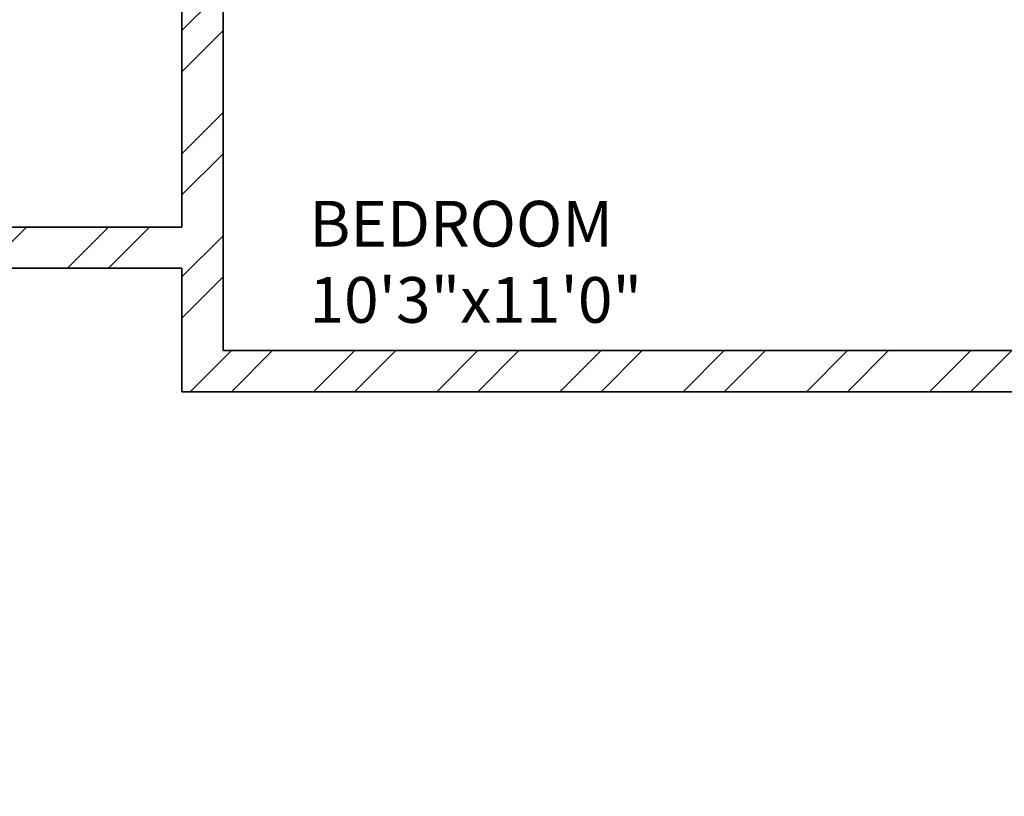
# Model space of a CAD drawing. Units: inches. Extents: x 1885 to 2748, y 783 to 2421.
# Tile 90 of 117: x 2341 to 2449, y 2167 to 2252. Entities that reach past the tile are written whole.
import ezdxf

# ---------------------------------------------------------------- set-up
doc = ezdxf.new("R2010")
doc.units = ezdxf.units.IN
doc.layers.add('A-AREA-IDEN', color=7, linetype='Continuous', lineweight=18)
doc.layers.add('A-WALL', color=7, linetype='Continuous', lineweight=35)
doc.layers.add('A-WALL-PATT', color=85, linetype='Continuous', lineweight=13, true_color=0x58ba48)
doc.styles.get("Standard").update_dxf_attribs({"font": 'arial.ttf'})

msp = doc.modelspace()

# ---------------------------------------------------------------- hatches: boundary and pattern name
at = {"layer": 'A-WALL-PATT'}
h = msp.add_hatch(dxfattribs=at)
h.set_pattern_fill('ANSI32', color=256)
h.paths.add_polyline_path([(2007.77, 2318.01), (1980.77, 2318.01), (1980.77, 2281.22), (1985.27, 2281.22), (1985.27, 2313.51), (2007.77, 2313.51), (2007.77, 2315.76)])
h.paths.add_polyline_path([(2094.32, 2318.01), (2067.77, 2318.01), (2067.77, 2313.51), (2094.32, 2313.51), (2094.32, 2315.76)])
h.paths.add_polyline_path([(2131.37, 2315.76), (2131.37, 2318.01), (2131.19, 2318.01), (2112.61, 2318.01), (2112.61, 2313.51), (2117.27, 2313.51), (2117.27, 2255.2), (2121.77, 2255.2), (2121.77, 2313.51), (2131.37, 2313.51)])
h.paths.add_polyline_path([(2190.51, 2318.01), (2155.37, 2318.01), (2155.37, 2313.51), (2169.77, 2313.51), (2169.77, 2229.51), (2121.77, 2229.51), (2121.77, 2233.45), (2119.52, 2233.45), (2117.27, 2233.45), (2117.27, 2201.1), (2121.77, 2201.1), (2121.77, 2225.01), (2169.77, 2225.01), (2169.77, 2165.01), (2306.27, 2165.01), (2306.27, 2066.01), (2310.77, 2066.01), (2344.27, 2066.01), (2486.27, 2066.01), (2486.27, 1886.01), (2483.02, 1886.01), (2483.02, 1881.51), (2486.27, 1881.51), (2486.27, 1880.68), (2490.77, 1880.68), (2490.77, 2070.51), (2344.27, 2070.51), (2310.77, 2070.51), (2310.77, 2165.01), (2310.77, 2173.64), (2308.52, 2173.64), (2306.27, 2173.64), (2306.27, 2169.51), (2174.27, 2169.51), (2174.27, 2313.51), (2190.51, 2313.51), (2190.51, 2315.76)])
h.paths.add_polyline_path([(1985.27, 2221.22), (1980.77, 2221.22), (1980.77, 2165.01), (1992.77, 2165.01), (1992.77, 2141.93), (1997.27, 2141.93), (1997.27, 2165.01), (2117.27, 2165.01), (2117.27, 2163.13), (2121.77, 2163.13), (2121.77, 2172.73), (2119.52, 2172.73), (2117.27, 2172.73), (2117.27, 2169.51), (1985.27, 2169.51)])
h.paths.add_polyline_path([(1997.27, 2105.93), (1992.77, 2105.93), (1992.77, 2070.51), (2016.77, 2070.51), (2016.77, 2059.12), (2019.02, 2059.12), (2021.27, 2059.12), (2021.27, 2070.51), (2117.27, 2070.51), (2117.27, 2022.51), (2114.42, 2022.51), (2114.42, 2018.01), (2123.63, 2018.01), (2123.63, 2020.26), (2123.63, 2022.51), (2121.77, 2022.51), (2121.77, 2142.59), (2119.52, 2142.59), (2117.27, 2142.59), (2117.27, 2075.01), (1997.27, 2075.01)])
h.paths.add_polyline_path([(2092.03, 2020.26), (2092.03, 2022.51), (2021.27, 2022.51), (2021.27, 2035.12), (2016.77, 2035.12), (2016.77, 2018.01), (2016.77, 1978.78), (2021.27, 1978.78), (2021.27, 2018.01), (2092.03, 2018.01)])
h.paths.add_polyline_path([(2260.94, 2022.51), (2153.1, 2022.51), (2153.1, 2020.26), (2153.1, 2018.01), (2155.27, 2018.01), (2155.27, 1886.01), (2107.63, 1886.01), (2107.63, 1881.51), (2182.91, 1881.51), (2182.91, 1883.76), (2182.91, 1886.01), (2159.77, 1886.01), (2159.77, 2018.01), (2260.94, 2018.01), (2260.94, 2020.26)])
h.paths.add_polyline_path([(2047.63, 1883.76), (2047.63, 1886.01), (2021.27, 1886.01), (2021.27, 1918.78), (2019.02, 1918.78), (2016.77, 1918.78), (2016.77, 1881.51), (2047.63, 1881.51)])
h.paths.add_polyline_path([(2306.36, 1883.76), (2306.36, 1886.01), (2296.27, 1886.01), (2296.27, 1982.01), (2316.54, 1982.01), (2316.54, 1984.26), (2316.54, 1986.51), (2296.27, 1986.51), (2296.27, 2022.51), (2289.28, 2022.51), (2289.28, 2018.01), (2291.77, 2018.01), (2291.77, 1886.01), (2242.91, 1886.01), (2242.91, 1881.51), (2306.36, 1881.51)], flags=17)
h.paths.add_polyline_path([(1985.27, 1843.01), (2021.6, 1843.01), (2021.53, 1845.44), (2021.48, 1847.51), (1980.77, 1847.51), (1980.77, 1809.45), (1985.27, 1809.45)])
h.paths.add_polyline_path([(2131.48, 1845.26), (2131.48, 1847.51), (2081.53, 1847.51), (2081.53, 1843.01), (2117.27, 1843.01), (2117.27, 1784.15), (2119.52, 1784.15), (2121.77, 1784.15), (2121.77, 1843.01), (2131.48, 1843.01)])
h.paths.add_polyline_path([(2203.89, 1847.51), (2155.48, 1847.51), (2155.48, 1843.01), (2169.77, 1843.01), (2169.77, 1759.01), (2121.77, 1759.01), (2121.77, 1761.46), (2117.27, 1761.46), (2117.27, 1730.43), (2121.77, 1730.43), (2121.77, 1754.51), (2177.42, 1754.51), (2177.42, 1756.76), (2177.42, 1759.01), (2174.27, 1759.01), (2174.27, 1843.01), (2203.89, 1843.01)])
h.paths.add_polyline_path([(2335.55, 1845.26), (2335.55, 1847.51), (2239.89, 1847.51), (2239.89, 1843.01), (2306.27, 1843.01), (2306.27, 1759.01), (2199.49, 1759.01), (2199.49, 1754.51), (2310.77, 1754.51), (2310.77, 1843.01), (2335.55, 1843.01)])
h.paths.add_polyline_path([(2348.77, 2022.51), (2344.27, 2022.51), (2344.27, 1986.51), (2341.68, 1986.51), (2341.68, 1982.01), (2344.27, 1982.01), (2344.27, 1886.01), (2330.36, 1886.01), (2330.36, 1881.51), (2361.63, 1881.51), (2361.63, 1883.76), (2361.63, 1886.01), (2348.77, 1886.01)], flags=17)
h.paths.add_polyline_path([(2283.25, 2315.76), (2283.25, 2318.01), (2238.51, 2318.01), (2238.51, 2313.51), (2283.25, 2313.51)], flags=17)
h.paths.add_polyline_path([(2363.27, 2348.01), (2388.68, 2348.01), (2388.68, 2350.26), (2388.68, 2352.51), (2358.77, 2352.51), (2358.77, 2348.01), (2358.77, 2318.01), (2344.48, 2318.01), (2344.48, 2313.51), (2358.77, 2313.51), (2358.77, 2229.51), (2310.77, 2229.51), (2310.77, 2231.95), (2306.27, 2231.95), (2306.27, 2205.61), (2310.77, 2205.61), (2310.77, 2225.01), (2358.77, 2225.01), (2358.77, 2211.51), (2452.33, 2211.51), (2452.33, 2213.76), (2452.33, 2216.01), (2363.27, 2216.01), (2363.27, 2318.01)])
h.paths.add_polyline_path([(2310.77, 2313.51), (2320.48, 2313.51), (2320.48, 2315.76), (2320.48, 2318.01), (2302.73, 2318.01), (2302.73, 2313.51), (2306.27, 2313.51), (2306.27, 2251.08), (2310.77, 2251.08)], flags=17)
h.paths.add_polyline_path([(2490.77, 2352.51), (2486.27, 2352.51), (2448.68, 2352.51), (2448.68, 2348.01), (2486.27, 2348.01), (2486.27, 2318.01), (2486.27, 2216.01), (2481.78, 2216.01), (2481.78, 2211.51), (2486.27, 2211.51), (2486.27, 2165.01), (2493.29, 2165.01), (2493.29, 2167.26), (2493.29, 2169.51), (2490.77, 2169.51), (2490.77, 2313.51), (2494.43, 2313.51), (2494.43, 2318.01), (2490.77, 2318.01)])
h.paths.add_polyline_path([(2534.65, 2318.01), (2515.69, 2318.01), (2515.69, 2313.51), (2534.65, 2313.51), (2534.65, 2315.76)])
h.paths.add_polyline_path([(2618.27, 2318.01), (2594.65, 2318.01), (2594.65, 2313.51), (2613.77, 2313.51), (2613.77, 2281.71), (2618.27, 2281.71)])
h.paths.add_polyline_path([(2618.27, 2221.71), (2613.77, 2221.71), (2613.77, 2169.51), (2554.02, 2169.51), (2554.02, 2165.01), (2613.77, 2165.01), (2613.77, 2152.88), (2618.27, 2152.88)])
h.paths.add_polyline_path([(2618.27, 2128.88), (2616.02, 2128.88), (2613.77, 2128.88), (2613.77, 2117.01), (2529.77, 2117.01), (2529.77, 2165.01), (2532.85, 2165.01), (2532.85, 2169.51), (2522.87, 2169.51), (2522.87, 2165.01), (2525.27, 2165.01), (2525.27, 2117.01), (2525.27, 2112.51), (2525.27, 2108.58), (2529.77, 2108.58), (2529.77, 2112.51), (2613.77, 2112.51), (2613.77, 2080.19), (2618.27, 2080.19)])
h.paths.add_polyline_path([(2618.27, 2044.19), (2616.02, 2044.19), (2613.77, 2044.19), (2613.77, 2015.51), (2529.77, 2015.51), (2529.77, 2088.58), (2527.52, 2088.58), (2525.27, 2088.58), (2525.27, 2011.01), (2613.77, 2011.01), (2613.77, 1956.75), (2618.27, 1956.75)])
h.paths.add_polyline_path([(2618.27, 1881.51), (2618.27, 1896.75), (2613.77, 1896.75), (2613.77, 1881.51), (2613.77, 1847.51), (2592.71, 1847.51), (2592.71, 1843.01), (2613.77, 1843.01), (2613.77, 1765.01), (2613.77, 1760.51), (2609.62, 1760.51), (2609.62, 1756.01), (2613.77, 1756.01), (2613.77, 1660.01), (2608.54, 1660.01), (2608.54, 1655.51), (2613.77, 1655.51), (2613.77, 1508.16), (2618.27, 1508.16)])
h.paths.add_polyline_path([(2565.77, 1843.01), (2569, 1843.01), (2569, 1847.51), (2490.77, 1847.51), (2490.77, 1849.7), (2488.52, 1849.7), (2486.27, 1849.7), (2486.27, 1847.51), (2477.27, 1847.51), (2477.27, 1838.51), (2477.27, 1821.49), (2486.27, 1821.49), (2486.27, 1838.51), (2561.27, 1838.51), (2561.27, 1765.01), (2486.27, 1765.01), (2486.27, 1786.16), (2477.27, 1786.16), (2477.27, 1765.01), (2477.27, 1756.01), (2486.27, 1756.01), (2565.77, 1756.01), (2585.62, 1756.01), (2585.62, 1758.26), (2585.62, 1760.51), (2565.77, 1760.51), (2565.77, 1765.01)])
h.paths.add_polyline_path([(2486.27, 1651.01), (2561.27, 1651.01), (2561.27, 1567.01), (2486.27, 1567.01), (2486.27, 1591.32), (2477.27, 1591.32), (2477.27, 1567.01), (2477.27, 1558.01), (2477.27, 1555.44), (2481.77, 1555.44), (2481.77, 1558.01), (2568.65, 1558.01), (2568.65, 1560.26), (2568.65, 1562.51), (2565.77, 1562.51), (2565.77, 1655.51), (2584.54, 1655.51), (2584.54, 1657.76), (2584.54, 1660.01), (2565.77, 1660.01), (2486.27, 1660.01), (2477.27, 1660.01), (2477.27, 1651.01), (2477.27, 1632.99), (2486.27, 1632.99)])
h.paths.add_polyline_path([(2449.97, 1883.76), (2449.97, 1886.01), (2421.63, 1886.01), (2421.63, 1881.51), (2449.97, 1881.51)], flags=17)
h.paths.add_polyline_path([(2447.27, 1847.51), (2395.55, 1847.51), (2395.55, 1843.01), (2442.77, 1843.01), (2442.77, 1809.27), (2447.27, 1809.27)])
h.paths.add_polyline_path([(1985.27, 1749.45), (1980.77, 1749.45), (1980.77, 1694.5), (1985.27, 1694.5), (1985.27, 1694.51), (1986.9, 1694.51), (1986.9, 1697.78), (1986.9, 1699.01), (1985.27, 1699.01)])
h.paths.add_polyline_path([(2152.77, 1699.01), (2121.77, 1699.01), (2121.77, 1703.67), (2119.52, 1703.67), (2117.27, 1703.67), (2117.27, 1699.01), (2009.22, 1699.01), (2009.22, 1694.51), (2148.27, 1694.51), (2148.27, 1692.63), (2152.77, 1692.63)])
h.paths.add_polyline_path([(2016.27, 1694.51), (2011.77, 1694.51), (2011.77, 1558.01), (2040.81, 1558.01), (2040.81, 1560.26), (2040.81, 1562.51), (2016.27, 1562.51)])
h.paths.add_polyline_path([(2152.77, 1663.02), (2150.52, 1663.02), (2148.27, 1663.02), (2148.27, 1562.51), (2100.81, 1562.51), (2100.81, 1558.01), (2165.12, 1558.01), (2165.12, 1560.26), (2165.12, 1562.51), (2152.77, 1562.51), (2152.77, 1610.51), (2224.77, 1610.51), (2224.77, 1607.99), (2229.27, 1607.99), (2229.27, 1615.01), (2152.77, 1615.01)])
h.paths.add_polyline_path([(2238.61, 1560.26), (2238.61, 1562.51), (2229.27, 1562.51), (2229.27, 1588.76), (2227.02, 1588.76), (2224.77, 1588.77), (2224.77, 1562.51), (2189.12, 1562.51), (2189.12, 1558.01), (2238.61, 1558.01)])
h.paths.add_polyline_path([(2336.02, 1560.26), (2336.02, 1562.51), (2310.77, 1562.51), (2310.77, 1656.35), (2308.52, 1656.35), (2306.27, 1656.35), (2306.27, 1562.51), (2286.61, 1562.51), (2286.61, 1558.01), (2336.02, 1558.01)])
h.paths.add_polyline_path([(2447.27, 1690.97), (2445.02, 1690.97), (2442.77, 1690.97), (2442.77, 1687.01), (2306.27, 1687.01), (2306.27, 1680.75), (2310.77, 1680.75), (2310.77, 1682.51), (2442.77, 1682.51), (2442.77, 1562.51), (2396.02, 1562.51), (2396.02, 1558.01), (2447.27, 1558.01)])
h.paths.add_polyline_path([(2447.27, 1749.27), (2445.02, 1749.27), (2442.77, 1749.27), (2442.77, 1717.23), (2447.27, 1717.23)])
h.paths.add_polyline_path([(2044.67, 1521.76), (2044.67, 1524.01), (2007.27, 1524.01), (2007.27, 1503.49), (2009.52, 1503.49), (2011.77, 1503.49), (2011.77, 1519.51), (2044.67, 1519.51)])
h.paths.add_polyline_path([(2177.97, 1521.76), (2177.97, 1524.01), (2104.67, 1524.01), (2104.67, 1519.51), (2145.77, 1519.51), (2145.77, 1387.51), (2143.37, 1387.51), (2143.37, 1383.01), (2251.59, 1383.01), (2251.59, 1385.26), (2251.59, 1387.51), (2150.27, 1387.51), (2150.27, 1519.51), (2177.97, 1519.51)])
h.paths.add_polyline_path([(2298.7, 1524.01), (2237.97, 1524.01), (2237.97, 1519.51), (2282.27, 1519.51), (2282.27, 1387.51), (2279.68, 1387.51), (2279.68, 1383.01), (2286.77, 1383.01), (2286.77, 1419.01), (2312.45, 1419.01), (2312.45, 1421.26), (2312.45, 1423.51), (2286.77, 1423.51), (2286.77, 1519.51), (2298.7, 1519.51), (2298.7, 1521.72)], flags=17)
h.paths.add_polyline_path([(2361.9, 1521.76), (2361.9, 1524.01), (2322.7, 1524.01), (2322.7, 1519.51), (2334.77, 1519.51), (2334.77, 1423.51), (2331.93, 1423.51), (2331.93, 1419.01), (2334.77, 1419.01), (2334.77, 1387.51), (2334.77, 1383.23), (2339.27, 1383.23), (2339.27, 1387.51), (2339.27, 1519.51), (2361.9, 1519.51)], flags=17)
h.paths.add_polyline_path([(2447.27, 1521.76), (2447.27, 1524.01), (2421.9, 1524.01), (2421.9, 1519.51), (2447.27, 1519.51)], flags=17)
h.paths.add_polyline_path([(2481.77, 1529.6), (2479.52, 1529.6), (2477.27, 1529.6), (2477.27, 1524.01), (2474.49, 1524.01), (2474.49, 1519.51), (2477.27, 1519.51), (2477.27, 1334.51), (2296.77, 1334.51), (2296.77, 1240.51), (2160.27, 1240.51), (2160.27, 1180.51), (2112.27, 1180.51), (2112.27, 1207.69), (2110.02, 1207.69), (2107.77, 1207.69), (2107.77, 1171.61), (2112.27, 1171.61), (2112.27, 1176.01), (2160.27, 1176.01), (2160.27, 1092.01), (2144.22, 1092.01), (2144.22, 1087.51), (2189.5, 1087.51), (2189.5, 1089.76), (2189.5, 1092.01), (2164.77, 1092.01), (2164.77, 1236.01), (2296.77, 1236.01), (2296.77, 1231.91), (2301.27, 1231.91), (2301.27, 1330.01), (2481.77, 1330.01), (2481.77, 1387.51)])
h.paths.add_polyline_path([(2618.27, 1448.16), (2613.77, 1448.16), (2613.77, 1382.51), (2529.77, 1382.51), (2525.27, 1382.51), (2525.27, 1307.06), (2529.77, 1307.06), (2529.77, 1378.01), (2613.77, 1378.01), (2613.77, 1354.99), (2618.27, 1354.99)])
h.paths.add_polyline_path([(2618.27, 1318.99), (2613.77, 1318.99), (2613.77, 1281.01), (2529.77, 1281.01), (2529.77, 1283.79), (2527.52, 1283.79), (2525.27, 1283.79), (2525.27, 1228.51), (2516.79, 1228.51), (2516.79, 1224.01), (2533.48, 1224.01), (2533.48, 1226.26), (2533.48, 1228.51), (2529.77, 1228.51), (2529.77, 1276.51), (2613.77, 1276.51), (2613.77, 1266.02), (2618.27, 1266.02)])
h.paths.add_polyline_path([(2618.27, 1134.96), (2613.77, 1134.96), (2613.77, 1092.01), (2594.54, 1092.01), (2594.54, 1087.51), (2618.27, 1087.51)])
h.paths.add_polyline_path([(2534.54, 1092.01), (2509.77, 1092.01), (2509.77, 1087.51), (2534.54, 1087.51), (2534.54, 1089.76)])
h.paths.add_polyline_path([(2481.27, 1224.01), (2484.12, 1224.01), (2484.12, 1226.26), (2484.12, 1228.51), (2476.77, 1228.51), (2476.77, 1198.51), (2471.61, 1198.51), (2471.61, 1194.01), (2476.77, 1194.01), (2476.77, 1062.01), (2436.89, 1062.01), (2436.89, 1057.51), (2476.77, 1057.51), (2481.27, 1057.51), (2481.27, 1062.01), (2481.27, 1087.51), (2485.35, 1087.51), (2485.35, 1089.76), (2485.35, 1092.01), (2481.27, 1092.01), (2481.27, 1117.51)])
h.paths.add_polyline_path([(2439.9, 1198.51), (2349.27, 1198.51), (2349.27, 1194.01), (2349.27, 1180.51), (2301.27, 1180.51), (2301.27, 1201.9), (2299.02, 1201.9), (2296.77, 1201.9), (2296.77, 1172.34), (2299.02, 1172.34), (2301.27, 1172.34), (2301.27, 1176.01), (2349.27, 1176.01), (2349.27, 1092.01), (2334.45, 1092.01), (2334.45, 1087.51), (2349.27, 1087.51), (2349.27, 1057.51), (2353.77, 1057.51), (2376.89, 1057.51), (2376.89, 1059.76), (2376.89, 1062.01), (2353.77, 1062.01), (2353.77, 1087.51), (2353.77, 1180.51), (2353.77, 1194.01), (2439.9, 1194.01), (2439.9, 1196.26)])
h.paths.add_polyline_path([(2270.6, 1089.76), (2270.6, 1092.01), (2249.5, 1092.01), (2249.5, 1087.51), (2270.6, 1087.51)], flags=17)
h.paths.add_polyline_path([(2310.45, 1092.01), (2301.27, 1092.01), (2301.27, 1153.29), (2296.77, 1153.29), (2296.77, 1092.01), (2293.79, 1092.01), (2293.79, 1087.51), (2310.45, 1087.51), (2310.45, 1089.76)], flags=17)
h.paths.add_polyline_path([(2112.27, 1150.33), (2110.02, 1150.33), (2107.77, 1150.33), (2107.77, 1092.01), (2104.47, 1092.01), (2104.47, 1087.51), (2120.22, 1087.51), (2120.22, 1089.76), (2120.22, 1092.01), (2112.27, 1092.01)])
h.paths.add_polyline_path([(2082.17, 1092.01), (2058.14, 1092.01), (2058.14, 1087.51), (2082.17, 1087.51), (2082.17, 1089.76)])
h.paths.add_polyline_path([(1975.77, 1145.64), (1971.27, 1145.64), (1971.27, 1087.51), (1980.77, 1087.51), (1998.14, 1087.51), (1998.14, 1089.76), (1998.14, 1092.01), (1985.27, 1092.01), (1975.77, 1092.01)])
h.paths.add_polyline_path([(2112.27, 1244.38), (2110.02, 1244.38), (2107.77, 1244.38), (2107.77, 1240.51), (1992.27, 1240.51), (1992.27, 1271.01), (1987.77, 1271.01), (1987.77, 1240.51), (1980.77, 1240.51), (1975.77, 1240.51), (1971.27, 1240.51), (1971.27, 1205.64), (1975.77, 1205.64), (1975.77, 1236.01), (2107.77, 1236.01), (2107.77, 1233.44), (2112.27, 1233.44), (2112.27, 1236.01)])
h.paths.add_polyline_path([(2112.27, 1383.01), (2114.78, 1383.01), (2114.78, 1385.26), (2114.78, 1387.51), (2102.48, 1387.51), (2102.48, 1383.01), (2107.77, 1383.01), (2107.77, 1335.01), (2011.77, 1335.01), (2011.77, 1349.94), (2007.27, 1349.94), (2007.27, 1335.01), (1987.77, 1335.01), (1987.77, 1330.51), (1987.77, 1307.01), (1992.27, 1307.01), (1992.27, 1330.51), (2007.27, 1330.51), (2107.77, 1330.51), (2107.77, 1264.71), (2112.27, 1264.71)])
h.paths.add_polyline_path([(2077.86, 1387.51), (2011.77, 1387.51), (2011.77, 1390.04), (2009.52, 1390.04), (2007.27, 1390.04), (2007.27, 1373.94), (2011.77, 1373.94), (2011.77, 1383.01), (2077.86, 1383.01)])
h.paths.add_polyline_path([(2011.77, 1443.49), (2007.27, 1443.49), (2007.27, 1410.25), (2011.77, 1410.25)])

# ---------------------------------------------------------------- linework, layer by layer
at = {"layer": 'A-WALL'}
for p, q in [((2363.27, 2318.01), (2363.27, 2216.01)), ((2358.77, 2313.51), (2358.77, 2229.51)), ((2310.77, 2229.51), (2358.77, 2229.51)), ((2310.77, 2225.01), (2358.77, 2225.01)), ((2358.77, 2225.01), (2358.77, 2211.51)), ((2363.27, 2216.01), (2453.64, 2216.01)), ((2358.77, 2211.51), (2452.33, 2211.51))]:
    msp.add_line(p, q, dxfattribs=at)

# ---------------------------------------------------------------- texts
at = {"layer": 'A-AREA-IDEN', "insert": (2372.7, 2232.39), "char_height": 5, "attachment_point": 1}
msp.add_mtext_dynamic_manual_height_columns('BEDROOM\\P10\'3"x11\'0"', width=122.2066, gutter_width=12.5, heights=[0], dxfattribs=at)

doc.saveas('drawing.dxf')
